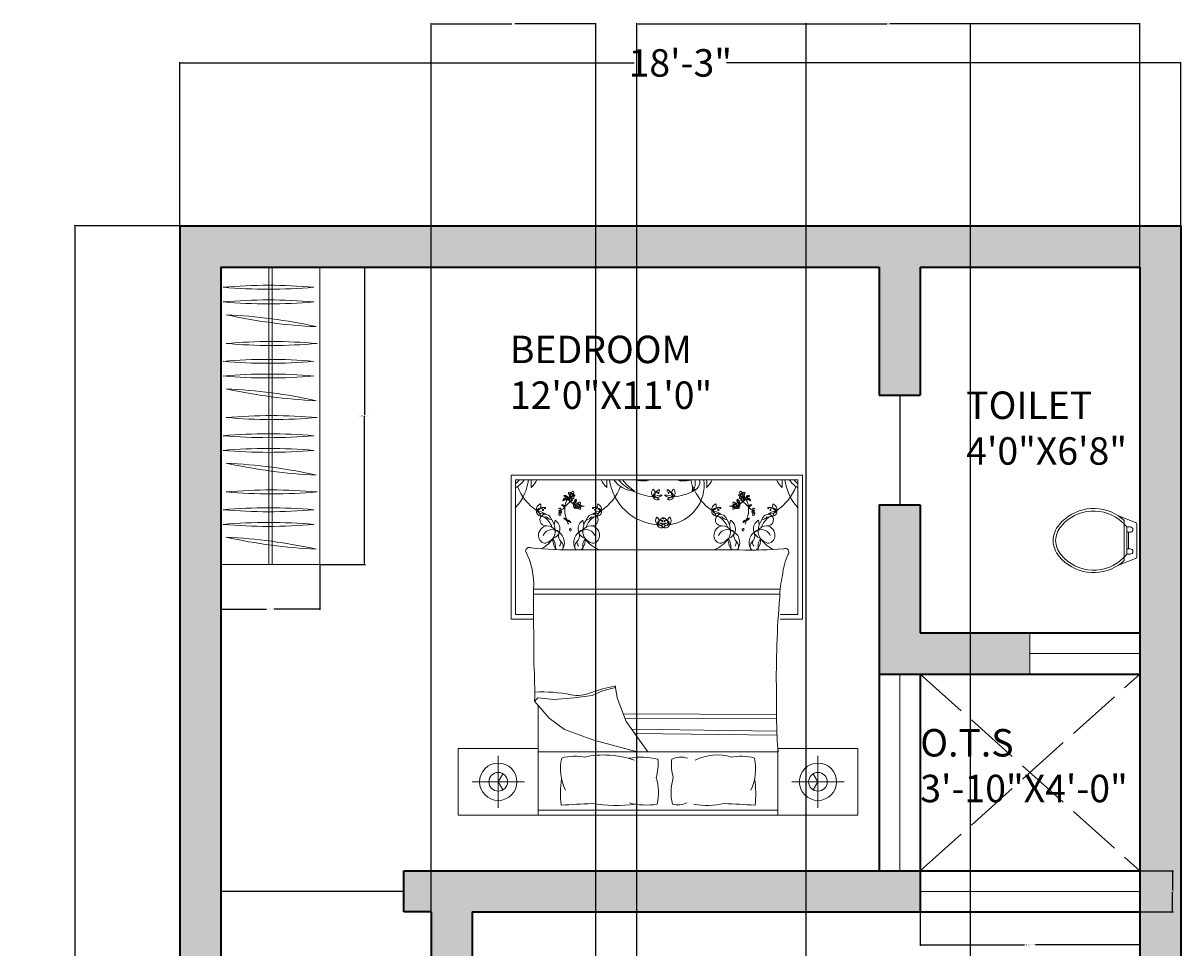
# Model space of a CAD drawing. Units: inches. Extents: x -16 to 587, y -783 to 64.
# Tile 12 of 14: x -16 to 237, y -138 to 64. Entities that reach past the tile are written whole.
import ezdxf

# ---------------------------------------------------------------- set-up
doc = ezdxf.new("R2010")
doc.units = ezdxf.units.IN
doc.header["$MEASUREMENT"] = 0
doc.linetypes.add('ACAD_ISO02W100', pattern=[15, 12, -3])
for name, color, linetype, lineweight in [('A-ANNO-DIMS', 2, 'Continuous', 18), ('A-AREA-IDEN', 7, 'Continuous', 18), ('A-DOOR', 3, 'Continuous', 25), ('A-FLOR-FIXT', 9, 'Continuous', 18), ('A-FLOR-OPEN', 8, 'ACAD_ISO02W100', 13), ('A-FURN', 8, 'Continuous', 18), ('A-GLAZ', 4, 'Continuous', 18), ('A-WALL', 7, 'Continuous', 35), ('A-WALL-PATT', 23, 'Continuous', 13)]:
    doc.layers.add(name, color=color, linetype=linetype, lineweight=lineweight)
doc.styles.get("Standard").update_dxf_attribs({"font": 'arial.ttf'})
doc.dimstyles.get("Standard").update_dxf_attribs({"dimtxt": 0.18, "dimasz": 0.18, "dimexe": 0.18, "dimexo": 0.0625, "dimgap": 0.09, "dimtad": 0, "dimtih": 1, "dimtoh": 1, "dimdec": 0, "dimzin": 0, "dimdsep": 46, "dimlunit": 3, "dimtxsty": 'Standard', "dimcen": 0.09, "dimadec": 0, "dimazin": 0, "dimtfac": 1, "dimtdec": 0, "dimtofl": 0, "dimtmove": 0, "dimatfit": 3, "dimfxl": 1, "dimtolj": 1, "dimtzin": 0, "dimarcsym": 0})

# ---------------------------------------------------------------- blocks, each defined once
blk = doc.blocks.new('*D5')
at = {"layer": 'A-ANNO-DIMS', "color": 0, "lineweight": -2, "transparency": 16777216}
for p, q in [((18.08, 19.51), (18.08, 55.27)), ((18.26, 55.09), (117.47, 55.09)), ((236.9, 55.09), (137.7, 55.09)), ((237.08, 19.51), (237.08, 55.27))]:
    blk.add_line(p, q, dxfattribs=at)
at = {"layer": 'A-ANNO-DIMS', "color": 0, "transparency": 16777216}
for points in [[(18.26, 55.12), (18.26, 55.06), (18.08, 55.09)], [(236.9, 55.12), (236.9, 55.06), (237.08, 55.09)]]:
    blk.add_solid(points, dxfattribs=at)
at = {"layer": 'Defpoints', "color": 0, "transparency": 16777216}
for p in [(237.08, 55.09), (18.08, 19.45), (237.08, 19.45)]:
    blk.add_point(p, dxfattribs=at)
at = {"layer": 'A-ANNO-DIMS', "color": 0, "transparency": 16777216, "insert": (127.58, 55.09), "char_height": 6, "attachment_point": 5}
blk.add_mtext('\\A1;18\'-3"', dxfattribs=at)
blk = doc.blocks.new('*D6')
at = {"layer": 'A-ANNO-DIMS', "color": 0, "lineweight": -2, "transparency": 16777216}
for p, q in [((18.02, 19.45), (-5.05, 19.45)), ((-4.87, 19.27), (-4.87, -355.9)), ((-4.87, -737.37), (-4.87, -362.21)), ((18.02, -737.55), (-5.05, -737.55))]:
    blk.add_line(p, q, dxfattribs=at)
at = {"layer": 'A-ANNO-DIMS', "color": 0, "transparency": 16777216}
for points in [[(-4.9, 19.27), (-4.84, 19.27), (-4.87, 19.45)], [(-4.9, -737.37), (-4.84, -737.37), (-4.87, -737.55)]]:
    blk.add_solid(points, dxfattribs=at)
at = {"layer": 'Defpoints', "color": 0, "transparency": 16777216}
for p in [(18.08, 19.45), (-4.87, -737.55), (18.08, -737.55)]:
    blk.add_point(p, dxfattribs=at)
at = {"layer": 'A-ANNO-DIMS', "color": 0, "transparency": 16777216, "insert": (-4.87, -359.05), "char_height": 6, "attachment_point": 5}
blk.add_mtext('\\A1;63\'-1"', dxfattribs=at)
blk = doc.blocks.new('BED-DOUBLE-LARGE')
for p, q in [((11.54, 74.35), (11.54, 42.86)), ((75.28, 74.35), (11.54, 74.35)), ((75.28, 42.86), (75.28, 74.35)), ((12.55, 73.34), (74.26, 73.34)), ((12.55, 43.87), (12.55, 73.34)), ((74.26, 73.34), (74.26, 43.87)), ((21.17, 64.47), (20.98, 63.49)), ((27.28, 64.47), (27.47, 63.49)), ((59.54, 64.47), (59.35, 63.49)), ((65.65, 64.47), (65.84, 63.49)), ((61.46, 57.99), (25.97, 57.99)), ((70.42, 49.4), (16.48, 49.4)), ((70.34, 48.31), (16.48, 48.31)), ((16.48, 43.87), (12.55, 43.87)), ((74.26, 43.87), (70.41, 43.87)), ((11.54, 42.86), (16.49, 42.86)), ((70.43, 42.86), (75.28, 42.86)), ((34.41, 27.92), (31.58, 27.21)), ((34.77, 25.62), (34.41, 27.92)), ((17.41, 25.62), (16.7, 24.91)), ((20.95, 25.26), (17.41, 25.62)), ((25.38, 25.62), (20.95, 25.26)), ((29.28, 26.15), (25.38, 25.62)), ((31.58, 27.21), (29.28, 26.15)), ((36.71, 20.49), (34.77, 25.62)), ((16.7, 24.91), (19.89, 21.19)), ((17.49, 0), (17.49, 24)), ((19.89, 21.19), (23.25, 18.72)), ((69.63, 22), (36.09, 22.13)), ((69.63, 21.1), (36.43, 21.23)), ((41.5, 13.82), (36.71, 20.49)), ((23.25, 18.72), (29.63, 16.41)), ((69.67, 18.35), (37.93, 18.79)), ((69.71, 17.45), (38.58, 17.88)), ((29.63, 16.41), (39.16, 13.82)), ((8.74, 13), (8.74, 1.57)), ((17.49, 13.82), (69.94, 13.82)), ((78.68, 13), (78.68, 1.57)), ((14.46, 7.29), (3.03, 7.29)), ((72.97, 7.29), (84.4, 7.29)), ((0, 0), (87.43, 0)), ((69.94, 1.12), (17.49, 1.12))]:
    blk.add_line(p, q)
for points in [[(16.52, 32.91, -0.001242), (16.48, 49.5, 0.127202), (14.73, 57.77)], [(70.32, 47.62, -0.056112), (70.95, 52.43, -0.095341), (72.18, 57.07)], [(22.51, 2.18, -0.074897), (22.61, 7.89, 0.472817)], [(43.3, 8.21, -0.14099), (43.48, 2.38, -0.235245)], [(47.04, 8.21, 0.14099), (46.86, 2.38, 0.235245)], [(64.92, 2.18, 0.074897), (64.81, 7.89, -0.472817)]]:
    blk.add_lwpolyline(points, format="xyb")
for points in [[(17.49, 14.57), (0, 14.57), (0, 0)], [(69.94, 0), (69.94, 14.57), (87.43, 14.57), (87.43, 0)], [(8.74, 7.29), (9.76, 9.05)], [(78.68, 7.29), (77.66, 9.05)], [(8.74, 7.29), (9.76, 5.52)], [(78.68, 7.29), (77.66, 5.52)]]:
    blk.add_lwpolyline(points)
for centre, radius in [((24.76, 69.99), 0.223), ((62.05, 69.99), 0.223), ((26.22, 67.64), 0.223), ((60.6, 67.64), 0.223), ((8.74, 7.29), 4.08), ((78.68, 7.29), 4.08), ((8.74, 7.29), 2.04), ((78.68, 7.29), 2.04)]:
    blk.add_circle(centre, radius)
for centre, radius, start, end in [((7.78, 77.44), 6.93, 313.5186, 323.6964), ((9.78, 76.41), 5.56, 299.8884, 326.5383), ((4.05, 74.88), 11.42, 318.1144, 352.255), ((23.59, 76.01), 11.42, 201.4092, 235.6135), ((12.9, 75.12), 4.64, 311.0454, 337.4453), ((0.18, 72.62), 15.8, 356.3481, 2.5919), ((35.55, 75.12), 4.64, 202.5547, 228.9546), ((24.86, 76.01), 11.42, 304.3865, 338.5908), ((48.27, 72.62), 15.8, 177.4081, 183.6519), ((44.39, 74.88), 11.42, 187.745, 265.5377), ((38.67, 76.41), 5.56, 213.4617, 268.728), ((40.67, 77.44), 6.93, 216.3036, 252.1496), ((44.31, 79.39), 10.31, 215.947, 235.9877), ((40.33, 79.34), 6.28, 252.9798, 286.4569), ((42.81, 82.58), 9.28, 264.3643, 265.6213), ((47.7, 88.94), 16.59, 250.0972, 250.2783), ((43.57, 70.46), 1.27, 140.8855, 222.2127), ((42.13, 70.42), 0.953, 301.6373, 61.4609), ((45.36, 68.67), 2.89, 121.989, 161.0841), ((43.91, 71), 0.142, 288.4408, 121.989), ((43.93, 70.93), 0.0689, 171.9833, 288.4408), ((45.82, 71), 0.142, 58.011, 251.5592), ((45.8, 70.93), 0.0689, 251.5592, 8.0167), ((44.37, 68.67), 2.89, 18.9159, 58.011), ((44.97, 72.24), 8.84, 278.1803, 7.1364), ((47.6, 70.42), 0.953, 118.5391, 238.3627), ((46.16, 70.46), 1.27, 317.7873, 39.1145), ((49.41, 79.34), 6.28, 253.5431, 287.0202), ((46.92, 82.58), 9.28, 274.3787, 275.6357), ((42.03, 88.94), 16.59, 289.7217, 289.9028), ((46.11, 71.43), 5.11, 353.3805, 21.883), ((50.8, 72.86), 2.05, 280.9261, 13.6102), ((49.26, 72.57), 2.59, 318.0951, 17.1391), ((61.96, 76.01), 11.42, 201.4092, 235.6135), ((38.55, 72.62), 15.8, 356.3481, 2.5919), ((51.27, 75.12), 4.64, 311.0454, 337.4453), ((73.92, 75.12), 4.64, 202.5547, 228.9546), ((63.23, 76.01), 11.42, 304.3865, 338.5908), ((86.64, 72.62), 15.8, 177.4081, 183.6519), ((82.76, 74.88), 11.42, 187.745, 221.8856), ((77.04, 76.41), 5.56, 213.4617, 240.1116), ((79.04, 77.44), 6.93, 216.3036, 226.4814), ((23.14, 68.85), 0.249, 123.0979, 213.1364), ((23.57, 68.49), 0.673, 92.3172, 160.5201), ((26.65, 63.38), 6.5, 121.1156, 124.8118), ((23.49, 68.75), 0.58, 82.6008, 147.1845), ((23.33, 69.66), 0.249, 55.6077, 145.6462), ((23.16, 69.13), 0.673, 21.7087, 93.0299), ((19.61, 64.33), 6.5, 53.6254, 57.3216), ((23.42, 68.72), 0.257, 45.7354, 121.1156), ((26.93, 67.08), 3.63, 150.7959, 175.244), ((32.15, 59.35), 11.95, 127.8256, 137.7588), ((23.36, 69.3), 0.58, 342.8042, 79.6943), ((23.31, 69.36), 0.257, 338.2452, 53.6254), ((23.73, 69.19), 0.194, 158.2452, 340.6395), ((23.74, 69.05), 0.194, 225.7354, 48.1297), ((27.39, 70.82), 3.88, 201.7087, 206.2181), ((24.3, 68.17), 1.01, 40.9365, 112.7695), ((23.96, 68.51), 0.597, 49.3812, 95.5456), ((26.93, 67.08), 3.63, 137.5083, 145.9967), ((24.4, 68.75), 0.617, 61.1838, 141.6792), ((27.3, 71.9), 4.35, 220.182, 239.456), ((24.3, 70.41), 0.221, 134.3732, 211.9501), ((24.7, 70.66), 0.702, 211.9501, 255.2442), ((24.31, 70.16), 0.439, 8.5614, 112.5914), ((24.52, 69.68), 0.304, 88.5719, 233.8954), ((24.48, 69.6), 0.218, 228.2946, 6.2474), ((24.82, 69.51), 0.718, 229.3812, 289.9959), ((24.43, 70.18), 0.147, 352.868, 97.094), ((24.28, 69.86), 0.306, 298.8493, 359.9355), ((24.35, 69.6), 0.35, 4.2123, 48.1587), ((25.07, 70.4), 0.368, 100.9597, 208.7804), ((25.07, 69.64), 0.371, 183.635, 258.4363), ((24.36, 68.63), 0.737, 15.6484, 62.2957), ((25.02, 69.78), 0.213, 178.1325, 268.8919), ((25.46, 69.91), 0.676, 132.3896, 156.5724), ((25.17, 69.83), 0.364, 42.3208, 130.2111), ((25.25, 70.21), 0.46, 226.3462, 279.6513), ((24.77, 69.35), 0.535, 7.4968, 71.2737), ((24.76, 70.6), 0.517, 291.6382, 4.947), ((25.16, 70.68), 0.729, 254.2829, 276.9148), ((25.1, 70.63), 0.171, 4.947, 127.5263), ((25.14, 69.38), 0.172, 215.0752, 14.7644), ((24.78, 69.11), 1.01, 287.889, 359.722), ((24.75, 68.64), 0.597, 305.1128, 351.2773), ((25.23, 68.74), 0.617, 271.4625, 339.4747), ((25.29, 69.94), 0.192, 279.6513, 42.3208), ((26.05, 68.44), 0.718, 110.6625, 171.2773), ((25.13, 68.8), 0.737, 338.3627, 25.0101), ((26.52, 68.05), 0.368, 100.9597, 208.7804), ((26.56, 68.28), 0.171, 4.947, 127.5263), ((43.52, 80.99), 11.42, 242.5854, 265.5377), ((43.56, 69.65), 0.934, 76.148, 182.2415), ((45.02, 61.99), 7.99, 92.7418, 107.407), ((43.37, 71.25), 1.8, 245.6899, 314.4589), ((42.58, 67.66), 1.95, 44.6273, 88.5415), ((43.54, 69.87), 0.946, 196.1963, 296.9726), ((43.76, 70.43), 0.123, 140.0755, 76.148), ((44.71, 61.99), 7.99, 72.593, 87.2582), ((46.36, 71.25), 1.8, 225.5411, 294.3101), ((47.15, 67.66), 1.95, 91.4585, 135.3727), ((46.19, 69.87), 0.946, 243.0274, 343.8037), ((45.96, 70.39), 0.0744, 103.9791, 39.8091), ((46.17, 69.65), 0.934, 357.7585, 103.852), ((46.21, 80.99), 11.42, 274.4623, 297.4146), ((60.26, 68.28), 0.171, 52.4737, 175.053), ((60.3, 68.05), 0.368, 331.2196, 79.0403), ((61.69, 68.8), 0.737, 154.9899, 201.6373), ((61.58, 68.74), 0.617, 200.5253, 268.5375), ((62.04, 69.11), 1.01, 180.278, 252.111), ((60.77, 68.44), 0.718, 8.7227, 69.3375), ((61.52, 69.94), 0.192, 137.6792, 260.3487), ((61.65, 69.83), 0.364, 49.7889, 137.6792), ((62.07, 68.64), 0.597, 188.7227, 234.8872), ((61.57, 70.21), 0.46, 260.3487, 313.6538), ((62.05, 69.35), 0.535, 108.7263, 172.5032), ((61.68, 69.38), 0.172, 165.2356, 324.9248), ((61.72, 70.63), 0.171, 52.4737, 175.053), ((62.06, 70.6), 0.517, 175.053, 248.3618), ((61.66, 70.68), 0.729, 263.0852, 285.7171), ((59.52, 71.9), 4.35, 300.544, 319.818), ((62.46, 68.63), 0.737, 117.7043, 164.3516), ((62.52, 68.17), 1.01, 67.2305, 139.0635), ((62, 69.51), 0.718, 250.0041, 310.6188), ((61.8, 69.78), 0.213, 271.1081, 1.8675), ((61.35, 69.91), 0.676, 23.4276, 47.6104), ((61.75, 70.4), 0.368, 331.2196, 79.0403), ((61.75, 69.64), 0.371, 281.5637, 356.365), ((54.66, 59.35), 11.95, 42.2412, 52.1744), ((62.51, 70.16), 0.439, 67.4086, 171.4386), ((62.47, 69.6), 0.35, 131.8413, 175.7877), ((62.33, 69.6), 0.218, 173.7526, 311.7054), ((62.42, 68.75), 0.617, 38.3208, 118.8162), ((62.54, 69.86), 0.306, 180.0645, 241.1507), ((62.38, 70.18), 0.147, 82.906, 187.132), ((62.11, 70.66), 0.702, 284.7558, 328.0499), ((62.3, 69.68), 0.304, 306.1046, 91.4281), ((62.85, 68.51), 0.597, 84.4544, 130.6188), ((59.89, 67.08), 3.63, 34.0033, 42.4917), ((62.52, 70.41), 0.221, 328.0499, 45.6268), ((63.45, 69.3), 0.58, 100.3057, 197.1958), ((63.08, 69.05), 0.194, 131.8703, 314.2646), ((63.08, 69.19), 0.194, 199.3605, 21.7548), ((59.43, 70.82), 3.88, 333.7819, 338.2913), ((63.66, 69.13), 0.673, 86.9701, 158.2913), ((59.89, 67.08), 3.63, 4.756, 29.2041), ((63.4, 68.72), 0.257, 58.8844, 134.2646), ((63.5, 69.36), 0.257, 126.3746, 201.7548), ((63.32, 68.75), 0.58, 32.8155, 97.3992), ((63.25, 68.49), 0.673, 19.4799, 87.6828), ((63.49, 69.66), 0.249, 34.3538, 124.3923), ((67.21, 64.33), 6.5, 122.6784, 126.3746), ((60.17, 63.38), 6.5, 55.1882, 58.8844), ((63.67, 68.85), 0.249, 326.8636, 56.9021), ((18.37, 66.85), 1.27, 110.9613, 192.2885), ((18.06, 66.36), 0.946, 166.272, 267.0484), ((17.11, 67.54), 0.953, 271.7131, 31.5367), ((19.04, 64.41), 2.89, 92.0648, 131.1598), ((17.96, 66.15), 0.934, 46.2238, 152.3173), ((15.41, 58.79), 7.99, 62.8176, 77.4827), ((18.6, 67.64), 1.8, 215.7657, 284.5347), ((16.12, 64.92), 1.95, 14.7031, 58.6173), ((18.53, 66.74), 0.123, 110.2817, 46.2238), ((18.92, 67.08), 0.0689, 142.0591, 258.5166), ((18.94, 67.15), 0.142, 258.5166, 92.0648), ((22.21, 66.73), 0.368, 100.9597, 142.2379), ((21.9, 66.32), 0.223, 273.2768, 86.7232), ((22.16, 66.11), 0.213, 178.1325, 268.8919), ((22.6, 66.24), 0.676, 132.3896, 156.5724), ((22.31, 66.16), 0.364, 42.3208, 130.2111), ((22.39, 66.54), 0.46, 226.3462, 279.6513), ((21.91, 65.68), 0.535, 7.4968, 71.2737), ((21.9, 66.93), 0.517, 291.6382, 4.947), ((22.3, 67.01), 0.729, 254.2829, 276.9148), ((22.24, 66.96), 0.171, 4.947, 127.5263), ((17.25, 73.06), 8.3, 307.9541, 316.8459), ((22.43, 66.27), 0.192, 279.6513, 42.3208), ((22.65, 65.38), 2.47, 82.8698, 91.6736), ((22.99, 68.05), 0.459, 205.5379, 258.6744), ((22.33, 66.49), 1.38, 59.344, 79.7412), ((22.03, 66.49), 1.4, 43.6929, 51.7899), ((22.89, 67.42), 0.42, 355.7131, 81.6568), ((22.66, 67.05), 0.733, 27.3659, 59.344), ((23.21, 67.53), 0.178, 202.5583, 304.2343), ((30.53, 66.9), 7.24, 176.1723, 196.4158), ((25.06, 67.54), 0.617, 3.8774, 87.1501), ((24.62, 67.78), 0.597, 352.0748, 38.2393), ((24.52, 67.31), 1.01, 343.6301, 55.4631), ((25.92, 67.6), 0.718, 172.0748, 232.6895), ((24.94, 67.52), 0.737, 318.342, 4.9894), ((25.75, 68.06), 0.221, 134.3732, 211.9501), ((27.3, 71.9), 4.35, 246.1523, 246.9499), ((26.16, 68.32), 0.702, 211.9501, 255.2442), ((25.77, 67.81), 0.439, 8.5614, 112.5914), ((25.97, 67.33), 0.304, 88.5719, 233.8954), ((25.94, 67.25), 0.218, 228.2946, 6.2474), ((25.89, 67.83), 0.147, 352.868, 97.094), ((25.73, 67.51), 0.306, 298.8493, 359.9355), ((25.81, 67.25), 0.35, 4.2123, 48.1587), ((26.53, 67.3), 0.371, 183.635, 258.4363), ((26.48, 67.43), 0.213, 178.1325, 268.8919), ((26.92, 67.57), 0.676, 132.3896, 156.5724), ((26.62, 67.48), 0.364, 42.3208, 130.2111), ((26.7, 67.86), 0.46, 226.3462, 279.6513), ((26.21, 68.25), 0.517, 291.6382, 4.947), ((26.23, 67.01), 0.535, 7.4968, 71.2737), ((26.62, 68.34), 0.729, 254.2829, 276.9148), ((26.59, 67.03), 0.172, 215.0752, 14.7644), ((26.75, 67.59), 0.192, 279.6513, 42.3208), ((27.3, 71.9), 4.35, 265.2415, 272.8929), ((29.51, 67.15), 0.142, 87.9352, 281.4834), ((29.84, 67.64), 1.8, 255.4653, 324.2343), ((33.04, 58.79), 7.99, 102.5173, 117.1824), ((29.41, 64.41), 2.89, 48.8402, 87.9352), ((29.52, 67.08), 0.0689, 281.4834, 37.9409), ((30.48, 66.15), 0.934, 27.6827, 133.7762), ((29.94, 66.69), 0.0744, 133.7729, 69.7333), ((31.34, 67.54), 0.953, 148.4633, 268.2869), ((30.39, 66.36), 0.946, 272.9516, 13.728), ((32.32, 64.92), 1.95, 121.3827, 165.2969), ((30.07, 66.85), 1.27, 347.7115, 69.0387), ((56.75, 66.85), 1.27, 110.9613, 192.2885), ((56.43, 66.36), 0.946, 166.272, 267.0484), ((55.48, 67.54), 0.953, 271.7131, 31.5367), ((57.41, 64.41), 2.89, 92.0648, 131.1598), ((56.34, 66.15), 0.934, 46.2238, 152.3173), ((54.49, 64.92), 1.95, 14.7031, 58.6173), ((56.97, 67.64), 1.8, 215.7657, 284.5347), ((53.78, 58.79), 7.99, 62.8176, 77.4827), ((56.9, 66.74), 0.123, 110.2817, 46.2238), ((57.3, 67.08), 0.0689, 142.0591, 258.5166), ((57.31, 67.15), 0.142, 258.5166, 92.0648), ((59.52, 71.9), 4.35, 267.1071, 274.7585), ((60.07, 67.59), 0.192, 137.6792, 260.3487), ((60.2, 67.48), 0.364, 49.7889, 137.6792), ((60.11, 67.86), 0.46, 260.3487, 313.6538), ((60.22, 67.03), 0.172, 165.2356, 324.9248), ((60.59, 67.01), 0.535, 108.7263, 172.5032), ((60.61, 68.25), 0.517, 175.053, 248.3618), ((60.2, 68.34), 0.729, 263.0852, 285.7171), ((60.34, 67.43), 0.213, 271.1081, 1.8675), ((59.9, 67.57), 0.676, 23.4276, 47.6104), ((60.29, 67.3), 0.371, 281.5637, 356.365), ((61.05, 67.81), 0.439, 67.4086, 171.4386), ((61.01, 67.25), 0.35, 131.8413, 175.7877), ((60.88, 67.25), 0.218, 173.7526, 311.7054), ((60.93, 67.83), 0.147, 82.906, 187.132), ((61.08, 67.51), 0.306, 180.0645, 241.1507), ((60.66, 68.32), 0.702, 284.7558, 328.0499), ((60.84, 67.33), 0.304, 306.1046, 91.4281), ((61.88, 67.52), 0.737, 175.0106, 221.658), ((61.76, 67.54), 0.617, 92.8499, 176.1226), ((61.07, 68.06), 0.221, 328.0499, 45.6268), ((59.52, 71.9), 4.35, 293.0501, 293.8477), ((62.3, 67.31), 1.01, 124.5369, 196.3699), ((60.89, 67.6), 0.718, 307.3105, 7.9252), ((62.2, 67.78), 0.597, 141.7607, 187.9252), ((56.28, 66.9), 7.24, 343.5842, 3.8277), ((63.93, 67.42), 0.42, 98.3432, 184.2869), ((64.16, 67.05), 0.733, 120.656, 152.6341), ((63.61, 67.53), 0.178, 235.7657, 337.4417), ((69.56, 73.06), 8.3, 223.1541, 232.0459), ((64.79, 66.49), 1.4, 128.2101, 136.3071), ((64.49, 66.49), 1.38, 100.2588, 120.656), ((64.17, 65.38), 2.47, 88.3264, 97.1302), ((63.83, 68.05), 0.459, 281.3256, 334.4621), ((64.38, 66.27), 0.192, 137.6792, 260.3487), ((64.51, 66.16), 0.364, 49.7889, 137.6792), ((64.43, 66.54), 0.46, 260.3487, 313.6538), ((64.9, 65.68), 0.535, 108.7263, 172.5032), ((64.58, 66.96), 0.171, 52.4737, 175.053), ((64.92, 66.93), 0.517, 175.053, 248.3618), ((64.52, 67.01), 0.729, 263.0852, 285.7171), ((64.66, 66.11), 0.213, 271.1081, 1.8675), ((64.21, 66.24), 0.676, 23.4276, 47.6104), ((64.61, 66.73), 0.368, 37.7621, 79.0403), ((64.91, 66.32), 0.223, 93.2768, 266.7232), ((67.88, 67.15), 0.142, 87.9352, 281.4834), ((71.41, 58.79), 7.99, 102.5173, 117.1824), ((68.22, 67.64), 1.8, 255.4653, 324.2343), ((67.78, 64.41), 2.89, 48.8402, 87.9352), ((67.89, 67.08), 0.0689, 281.4834, 37.9409), ((68.85, 66.15), 0.934, 27.6827, 133.7762), ((68.31, 66.69), 0.0744, 133.7729, 69.7333), ((69.71, 67.54), 0.953, 148.4633, 268.2869), ((70.7, 64.92), 1.95, 121.3827, 165.2969), ((68.76, 66.36), 0.946, 272.9516, 13.728), ((68.44, 66.85), 1.27, 347.7115, 69.0387), ((19.17, 64.55), 1.31, 109.1312, 279.736), ((18.9, 65.97), 0.804, 216.7319, 296.0245), ((16.57, 61.66), 4.13, 18.2955, 58.7386), ((18.85, 64.15), 1.64, 15.6955, 94.031), ((20.62, 66.33), 1.75, 218.4175, 263.8338), ((16.53, 61.99), 4.69, 3.4924, 33.7117), ((20.08, 62.59), 2.17, 286.8663, 60.0915), ((22.21, 65.97), 0.371, 217.3642, 258.4363), ((22.28, 65.71), 0.172, 215.0752, 14.7644), ((23.17, 62.44), 2.47, 82.8698, 91.6736), ((23.51, 65.1), 0.459, 205.5379, 258.6744), ((22.85, 63.55), 1.38, 59.344, 79.7412), ((22.55, 63.55), 1.4, 43.6929, 51.7899), ((23.41, 64.47), 0.42, 355.7131, 81.6568), ((23.18, 64.11), 0.733, 27.3659, 59.344), ((23.73, 64.59), 0.178, 202.5583, 304.2343), ((30.53, 66.9), 7.24, 200.1059, 206.9968), ((24.06, 64.09), 0.42, 36.5232, 122.4668), ((23.84, 63.71), 0.733, 58.836, 90.8141), ((24.01, 64.42), 0.178, 173.9457, 275.6216), ((23.65, 62.89), 1.4, 66.3901, 74.4871), ((24.57, 64.47), 0.459, 219.5056, 272.6421), ((23.5, 63.15), 1.38, 38.4388, 58.836), ((22.38, 62.91), 2.47, 26.5064, 35.3102), ((28.36, 62.59), 2.17, 119.9085, 253.1337), ((31.92, 61.99), 4.69, 146.2883, 176.5076), ((31.88, 61.66), 4.13, 121.2614, 161.7045), ((29.59, 64.15), 1.64, 85.969, 164.3045), ((27.83, 66.33), 1.75, 276.1662, 321.5825), ((29.28, 64.55), 1.31, 260.264, 70.8688), ((29.55, 65.97), 0.804, 243.9755, 323.2681), ((44.44, 64.35), 1.27, 140.8855, 222.2127), ((43.01, 64.31), 0.953, 301.6373, 61.4609), ((44.44, 63.53), 0.934, 76.148, 182.2415), ((46.24, 62.56), 2.89, 121.989, 161.0841), ((44.25, 65.14), 1.8, 245.6899, 314.4589), ((45.89, 55.87), 7.99, 92.7418, 107.407), ((44.41, 63.76), 0.946, 196.1963, 296.9726), ((43.46, 61.55), 1.95, 44.6273, 88.5415), ((45.48, 65.14), 1.8, 225.5411, 294.3101), ((43.84, 55.87), 7.99, 72.593, 87.2582), ((44.63, 64.32), 0.123, 140.0755, 76.148), ((44.78, 64.89), 0.142, 288.4408, 121.989), ((44.81, 64.82), 0.0689, 171.9833, 288.4408), ((44.95, 64.89), 0.142, 58.011, 251.5592), ((45.32, 63.76), 0.946, 243.0274, 343.8037), ((46.28, 61.55), 1.95, 91.4585, 135.3727), ((44.93, 64.82), 0.0689, 251.5592, 8.0167), ((45.09, 64.27), 0.0744, 103.9791, 39.8091), ((43.5, 62.56), 2.89, 18.9159, 58.011), ((45.29, 63.53), 0.934, 357.7585, 103.852), ((46.73, 64.31), 0.953, 118.5391, 238.3627), ((45.29, 64.35), 1.27, 317.7873, 39.1145), ((57.54, 64.55), 1.31, 109.1312, 279.736), ((57.27, 65.97), 0.804, 216.7319, 296.0245), ((54.94, 61.66), 4.13, 18.2955, 58.7386), ((57.22, 64.15), 1.64, 15.6955, 94.031), ((58.99, 66.33), 1.75, 218.4175, 263.8338), ((54.9, 61.99), 4.69, 3.4924, 33.7117), ((58.46, 62.59), 2.17, 286.8663, 60.0915), ((63.31, 63.15), 1.38, 121.164, 141.5612), ((64.44, 62.91), 2.47, 144.6898, 153.4936), ((62.25, 64.47), 0.459, 267.3579, 320.4944), ((62.76, 64.09), 0.42, 57.5332, 143.4768), ((62.98, 63.71), 0.733, 89.1859, 121.164), ((63.17, 62.89), 1.4, 105.5129, 113.6099), ((56.28, 66.9), 7.24, 333.0032, 339.8941), ((62.81, 64.42), 0.178, 264.3784, 6.0543), ((63.41, 64.47), 0.42, 98.3432, 184.2869), ((63.64, 64.11), 0.733, 120.656, 152.6341), ((63.09, 64.59), 0.178, 235.7657, 337.4417), ((64.27, 63.55), 1.4, 128.2101, 136.3071), ((63.97, 63.55), 1.38, 100.2588, 120.656), ((63.65, 62.44), 2.47, 88.3264, 97.1302), ((63.31, 65.1), 0.459, 281.3256, 334.4621), ((64.54, 65.71), 0.172, 165.2356, 324.9248), ((66.73, 62.59), 2.17, 119.9085, 253.1337), ((64.61, 65.97), 0.371, 281.5637, 322.6358), ((70.29, 61.99), 4.69, 146.2883, 176.5076), ((70.25, 61.66), 4.13, 121.2614, 161.7045), ((67.96, 64.15), 1.64, 85.969, 164.3045), ((66.2, 66.33), 1.75, 276.1662, 321.5825), ((67.65, 64.55), 1.31, 260.264, 70.8688), ((67.92, 65.97), 0.804, 243.9755, 323.2681), ((19.65, 61.18), 2.09, 97.1143, 185.0551), ((19.04, 60.97), 1.48, 178.9462, 275.5144), ((20.47, 60.39), 2.03, 68.5779, 158.4181), ((18.59, 62.06), 2.63, 283.079, 4.7067), ((19.29, 60.71), 2.54, 35.9599, 87.6409), ((24.06, 60.21), 3.37, 143.6555, 147.2989), ((21.46, 61.68), 0.543, 344.8529, 102.6959), ((20.42, 59.58), 2.79, 330.8249, 70.7178), ((23.71, 61.07), 1.79, 164.8529, 228.4347), ((24.47, 62.5), 0.169, 79.5616, 257.2949), ((24.46, 62.4), 0.274, 259.5864, 79.5616), ((28.03, 59.58), 2.79, 109.2822, 209.1751), ((24.73, 61.07), 1.79, 311.5653, 15.1471), ((26.99, 61.68), 0.543, 77.3041, 195.1471), ((29.16, 60.71), 2.54, 92.3591, 144.0401), ((24.39, 60.21), 3.37, 32.7011, 36.3445), ((29.86, 62.06), 2.63, 175.2933, 256.921), ((27.98, 60.39), 2.03, 21.5819, 111.4221), ((28.8, 61.18), 2.09, 354.9449, 82.8857), ((29.4, 60.97), 1.48, 264.4856, 1.0538), ((58.02, 61.18), 2.09, 97.1143, 185.0551), ((57.41, 60.97), 1.48, 178.9462, 275.5144), ((58.84, 60.39), 2.03, 68.5779, 158.4181), ((56.96, 62.06), 2.63, 283.079, 4.7067), ((57.66, 60.71), 2.54, 35.9599, 87.6409), ((62.43, 60.21), 3.37, 143.6555, 147.2989), ((59.83, 61.68), 0.543, 344.8529, 102.6959), ((58.79, 59.58), 2.79, 330.8249, 70.7178), ((62.09, 61.07), 1.79, 164.8529, 228.4347), ((62.36, 62.4), 0.274, 100.4384, 280.4136), ((62.34, 62.5), 0.169, 282.7051, 100.4384), ((66.4, 59.58), 2.79, 109.2822, 209.1751), ((63.1, 61.07), 1.79, 311.5653, 15.1471), ((65.36, 61.68), 0.543, 77.3041, 195.1471), ((67.53, 60.71), 2.54, 92.3591, 144.0401), ((62.76, 60.21), 3.37, 32.7011, 36.3445), ((68.23, 62.06), 2.63, 175.2933, 256.921), ((66.35, 60.39), 2.03, 21.5819, 111.4221), ((67.17, 61.18), 2.09, 354.9449, 82.8857), ((67.77, 60.97), 1.48, 264.4856, 1.0538), ((15.53, 57.71), 0.807, 62.6588, 176.02), ((24.92, 148.99), 91.01, 264.3113, 270.6567), ((15.19, 64.15), 6.62, 296.7003, 326.3329), ((24.06, 60.21), 3.37, 175.2696, 214.215), ((17.62, 58.64), 3.62, 350.8446, 31.1782), ((22.1, 58.96), 1.05, 217.675, 239.9707), ((20, 60.08), 2.51, 330.0851, 352.564), ((21.66, 58.75), 1.31, 336.1646, 48.4347), ((26.79, 58.75), 1.31, 131.5653, 203.8354), ((28.45, 60.08), 2.51, 187.436, 209.9149), ((26.34, 58.96), 1.05, 293.2856, 322.325), ((24.39, 60.21), 3.37, 325.785, 4.7304), ((30.83, 58.64), 3.62, 148.8218, 190.2867), ((33.26, 64.15), 6.62, 213.6671, 248.5059), ((53.56, 64.15), 6.62, 291.4941, 326.3329), ((62.43, 60.21), 3.37, 175.2696, 214.215), ((55.99, 58.64), 3.62, 349.7133, 31.1782), ((60.47, 58.96), 1.05, 217.675, 246.7144), ((58.37, 60.08), 2.51, 330.0851, 352.564), ((60.03, 58.75), 1.31, 336.1646, 48.4347), ((65.16, 58.75), 1.31, 131.5653, 203.8354), ((66.82, 60.08), 2.51, 187.436, 209.9149), ((64.72, 58.96), 1.05, 287.4186, 322.325), ((62.76, 60.21), 3.37, 325.785, 4.7304), ((69.2, 58.64), 3.62, 148.8218, 190.751), ((71.63, 64.15), 6.62, 213.6671, 246.3547), ((71.52, 57.51), 0.797, 326.1736, 113.4781), ((22.1, 58.96), 1.05, 296.442, 315.5483), ((26.34, 58.96), 1.05, 224.4517, 246.771), ((60.47, 58.96), 1.05, 293.2856, 315.5483), ((64.14, 143.02), 85.07, 268.1965, 274.7598), ((64.72, 58.96), 1.05, 224.4517, 253.3657), ((274.49, 30.21), 204.92, 175.1265, 180.8855), ((-63.46, 27.08), 80.19, 358.447, 4.1706), ((40.48, -5.12), 33.91, 100.6617, 109.8806), ((34.21, 27.99), 0.211, 340.2464, 91.1377), ((18.2, -6.05), 33, 78.6608, 92.5481), ((26.09, 33.28), 7.12, 258.6608, 293.7384), ((226.67, 24.5), 157.09, 179.0718, 183.9), ((25.63, 1.16), 11.72, 78.9631, 104.8961), ((31.79, -7.17), 20.32, 70.7385, 101.9603), ((40.02, -2.74), 15.42, 76.3762, 100.1383), ((48.65, 8.05), 4.63, 71.4593, 114.9817), ((56.75, 2.02), 11.13, 73.8254, 116.1239), ((61.8, 1.16), 11.72, 75.1039, 101.0369), ((33.65, 10.18), 11.27, 168.2417, 204.8684), ((33, 11.13), 10.71, 344.1707, 5.9871), ((57.34, 11.13), 10.71, 174.0129, 195.8293), ((53.78, 10.18), 11.27, 335.1316, 11.7583), ((70.7, -829.84), 833.41, 92.85022, 93.31479), ((34.49, 33.82), 31.71, 260.503, 277.7804), ((41.18, 17.79), 15.58, 256.04, 278.4751), ((48.06, 6.54), 4.32, 253.8974, 296.6563), ((54.54, 17.48), 15.37, 258.8159, 283.6573), ((16.73, -829.84), 833.41, 86.68521, 87.14978)]:
    blk.add_arc(centre, radius, start, end)
blk = doc.blocks.new('WARDROBE')
for p, q in [((0, 0), (0, 65.01)), ((21.67, 65.01), (0, 65.01)), ((10.47, 0), (10.47, 65.01)), ((11.19, 0), (11.19, 65.01)), ((21.67, 0), (21.67, 65.01)), ((21.67, 0), (0, 0))]:
    blk.add_line(p, q)
for centre, start, end in [((10.4, -52.98), 85.0028, 94.9972), ((10.4, 174.18), 265.0028, 274.9972), ((10.4, -56.19), 85.0028, 94.9972), ((10.4, 170.97), 265.0028, 274.9972), ((25.83, 165.89), 257.508, 267.5023), ((-3.8, -59.33), 77.508, 87.5023), ((11.1, -65.28), 85.0028, 94.9972), ((11.1, 161.88), 265.0028, 274.9972), ((10.4, -69.18), 85.0028, 94.9972), ((10.4, 157.98), 265.0028, 274.9972), ((10.4, -72.39), 85.0028, 94.9972), ((10.4, 154.77), 265.0028, 274.9972), ((25.83, 149.7), 257.508, 267.5023), ((-3.8, -75.52), 77.508, 87.5023), ((11.1, -81.47), 85.0028, 94.9972), ((11.1, 145.69), 265.0028, 274.9972), ((10.4, -85.44), 85.0028, 94.9972), ((10.4, 141.72), 265.0028, 274.9972), ((10.4, -88.65), 85.0028, 94.9972), ((10.4, 138.51), 265.0028, 274.9972), ((-3.8, -91.78), 77.508, 87.5023), ((25.83, 133.44), 257.508, 267.5023), ((11.1, -97.73), 85.0028, 94.9972), ((11.1, 129.43), 265.0028, 274.9972), ((10.4, -101.63), 85.0028, 94.9972), ((10.4, 125.53), 265.0028, 274.9972), ((10.4, -104.84), 85.0028, 94.9972), ((10.4, 122.32), 265.0028, 274.9972), ((-3.8, -107.97), 77.508, 87.5023), ((25.83, 117.25), 257.508, 267.5023)]:
    blk.add_arc(centre, 114.01, start, end)
blk = doc.blocks.new('WC-PLAN')
for p, q in [((15.58, 11.39), (15.58, 10.62)), ((15.58, 10.62), (15.58, 7.01)), ((15.58, 3.4), (15.58, 7.01)), ((15.58, 3.4), (15.58, 2.63))]:
    blk.add_line(p, q)
for points in [[(14.32, 12.39, 0.383919), (1.32, 10.46, 0.163732), (0, 7.01, 0.359733)], [(15.2, 10.99, 0.431639), (1.75, 10.11, 0.162618), (0.55, 7.01, 0.470877)], [(15.58, 11.39, 0.040937), (14.32, 12.39, 0.163732)], [(18.36, 7.01), (18.36, 10.52, 0.31031), (18.06, 10.95), (14.32, 12.39, 0.209071)], [(15.58, 10.62, 0.014165), (15.2, 10.99, 0.162618)], [(16.13, 9.99, 0.022712), (15.58, 10.62, 0.162618)], [(16.13, 7.01), (16.13, 9.99, 0.022712)], [(16.13, 9.99), (16.9, 9.99, -1), (16.9, 8.82), (16.5, 8.82)], [(14.32, 1.64, -0.383919), (1.32, 3.56, -0.163732), (0, 7.01, -0.359733)], [(15.58, 3.4, -0.448546), (1.75, 3.91, -0.162618), (0.55, 7.01, -0.470877)], [(18.36, 7.01), (18.36, 3.51, -0.31031), (18.06, 3.08), (14.32, 1.64, -0.209071)], [(16.13, 7.01), (16.13, 4.03, -0.476108)], [(16.13, 4.03), (16.9, 4.03, 1), (16.9, 5.21), (16.5, 5.21)], [(15.58, 2.63, -0.040937), (14.32, 1.64, -0.163732)], [(16.13, 4.03, -0.022712), (15.58, 3.4, -0.162618)]]:
    blk.add_lwpolyline(points, format="xyb")
for points in [[(16.5, 8.82), (16.13, 8.82)], [(16.5, 5.21), (16.5, 8.82)], [(16.5, 5.21), (16.13, 5.21)]]:
    blk.add_lwpolyline(points)
blk = doc.blocks.new('WIN-24')
for p, q in [((0, 9), (0, 0)), ((0, 9), (24, 9)), ((24, 9), (24, 0)), ((0, 4.5), (24, 4.5)), ((24, 0), (0, 0))]:
    blk.add_line(p, q)
blk = doc.blocks.new('WIN-48')
for p, q in [((0, 9), (0, 0)), ((48, 9), (0, 9)), ((48, 0), (48, 9)), ((0, 4.5), (48, 4.5)), ((0, 0), (48, 0))]:
    blk.add_line(p, q)
blk = doc.blocks.new('*D28')
at = {"layer": 'A-ANNO-DIMS', "color": 0, "lineweight": -2, "transparency": 16777216}
for p, q in [((48.81, 10.45), (58.68, 10.45)), ((58.5, 10.27), (58.5, -21.87)), ((58.5, -54.38), (58.5, -22.24)), ((48.81, -54.56), (58.68, -54.56))]:
    blk.add_line(p, q, dxfattribs=at)
at = {"layer": 'A-ANNO-DIMS', "color": 0, "transparency": 16777216}
for points in [[(58.47, 10.27), (58.53, 10.27), (58.5, 10.45)], [(58.47, -54.38), (58.53, -54.38), (58.5, -54.56)]]:
    blk.add_solid(points, dxfattribs=at)
at = {"layer": 'Defpoints', "color": 0, "transparency": 16777216}
for p in [(48.75, 10.45), (58.5, 10.45), (48.75, -54.56)]:
    blk.add_point(p, dxfattribs=at)
at = {"layer": 'A-ANNO-DIMS', "color": 0, "transparency": 16777216, "insert": (58.5, -22.06), "char_height": 0.18, "attachment_point": 5}
blk.add_mtext('\\A1;WARDROBE 5\'-5" TYP.', dxfattribs=at)
blk = doc.blocks.new('*D29')
at = {"layer": 'A-ANNO-DIMS', "color": 0, "lineweight": -2, "transparency": 16777216}
for p, q in [((27.08, -54.62), (27.08, -64.49)), ((48.75, -54.62), (48.75, -64.49)), ((27.26, -64.31), (37.08, -64.31)), ((48.57, -64.31), (38.76, -64.31))]:
    blk.add_line(p, q, dxfattribs=at)
at = {"layer": 'A-ANNO-DIMS', "color": 0, "transparency": 16777216}
for points in [[(27.26, -64.28), (27.26, -64.34), (27.08, -64.31)], [(48.57, -64.28), (48.57, -64.34), (48.75, -64.31)]]:
    blk.add_solid(points, dxfattribs=at)
at = {"layer": 'Defpoints', "color": 0, "transparency": 16777216}
for p in [(27.08, -54.56), (48.75, -54.56), (48.75, -64.31)]:
    blk.add_point(p, dxfattribs=at)
at = {"layer": 'A-ANNO-DIMS', "color": 0, "transparency": 16777216, "insert": (37.92, -64.31), "char_height": 0.18, "attachment_point": 5}
blk.add_mtext('\\A1;1\'-9 1/2" TYP.', dxfattribs=at)
blk = doc.blocks.new('*D44')
at = {"layer": 'A-ANNO-DIMS', "color": 0, "lineweight": -2, "transparency": 16777216}
for p, q in [((180.08, -130.62), (180.08, -137.93)), ((228.08, -130.62), (228.08, -137.93)), ((180.26, -137.75), (202.85, -137.75)), ((227.9, -137.75), (205.31, -137.75))]:
    blk.add_line(p, q, dxfattribs=at)
at = {"layer": 'A-ANNO-DIMS', "color": 0, "transparency": 16777216}
for points in [[(180.26, -137.72), (180.26, -137.78), (180.08, -137.75)], [(227.9, -137.72), (227.9, -137.78), (228.08, -137.75)]]:
    blk.add_solid(points, dxfattribs=at)
at = {"layer": 'Defpoints', "color": 0, "transparency": 16777216}
for p in [(180.08, -130.55), (228.08, -130.55), (228.08, -137.75)]:
    blk.add_point(p, dxfattribs=at)
at = {"layer": 'A-ANNO-DIMS', "color": 0, "transparency": 16777216, "insert": (204.08, -137.75), "char_height": 0.18, "attachment_point": 5}
blk.add_mtext('\\A1;WINDOW 4\'-0" TYP.', dxfattribs=at)
blk = doc.blocks.new('*D45')
at = {"layer": 'A-ANNO-DIMS', "color": 0, "lineweight": -2, "transparency": 16777216}
for p, q in [((228.15, -121.55), (235.46, -121.55)), ((235.28, -121.73), (235.28, -125.87)), ((235.28, -130.37), (235.28, -126.24)), ((228.15, -130.55), (235.46, -130.55))]:
    blk.add_line(p, q, dxfattribs=at)
at = {"layer": 'A-ANNO-DIMS', "color": 0, "transparency": 16777216}
for points in [[(235.25, -121.73), (235.31, -121.73), (235.28, -121.55)], [(235.25, -130.37), (235.31, -130.37), (235.28, -130.55)]]:
    blk.add_solid(points, dxfattribs=at)
at = {"layer": 'Defpoints', "color": 0, "transparency": 16777216}
for p in [(228.08, -121.55), (235.28, -121.55), (228.08, -130.55)]:
    blk.add_point(p, dxfattribs=at)
at = {"layer": 'A-ANNO-DIMS', "color": 0, "transparency": 16777216, "insert": (235.28, -126.05), "char_height": 0.18, "attachment_point": 5}
blk.add_mtext('\\A1;0\'-9" TYP.', dxfattribs=at)
blk = doc.blocks.new('*D56')
at = {"layer": 'A-ANNO-DIMS', "color": 0, "lineweight": -2, "transparency": 16777216}
for p, q in [((118.08, -728.49), (118.08, 63.78)), ((118.26, 63.6), (172.75, 63.6)), ((227.9, 63.6), (173.41, 63.6)), ((228.08, -728.49), (228.08, 63.78))]:
    blk.add_line(p, q, dxfattribs=at)
at = {"layer": 'A-ANNO-DIMS', "color": 0, "transparency": 16777216}
for points in [[(118.26, 63.63), (118.26, 63.57), (118.08, 63.6)], [(227.9, 63.63), (227.9, 63.57), (228.08, 63.6)]]:
    blk.add_solid(points, dxfattribs=at)
at = {"layer": 'Defpoints', "color": 0, "transparency": 16777216}
for p in [(228.08, 63.6), (118.08, -728.55), (228.08, -728.55)]:
    blk.add_point(p, dxfattribs=at)
at = {"layer": 'A-ANNO-DIMS', "color": 0, "transparency": 16777216, "insert": (173.08, 63.6), "char_height": 0.18, "attachment_point": 5}
blk.add_mtext('\\A1;9\'-2"', dxfattribs=at)
blk = doc.blocks.new('*D57')
at = {"layer": 'A-ANNO-DIMS', "color": 0, "lineweight": -2, "transparency": 16777216}
for p, q in [((155.08, -534.49), (155.08, 63.78)), ((155.26, 63.6), (172.75, 63.6)), ((190.9, 63.6), (173.41, 63.6)), ((191.08, -534.49), (191.08, 63.78))]:
    blk.add_line(p, q, dxfattribs=at)
at = {"layer": 'A-ANNO-DIMS', "color": 0, "transparency": 16777216}
for points in [[(155.26, 63.63), (155.26, 63.57), (155.08, 63.6)], [(190.9, 63.63), (190.9, 63.57), (191.08, 63.6)]]:
    blk.add_solid(points, dxfattribs=at)
at = {"layer": 'Defpoints', "color": 0, "transparency": 16777216}
for p in [(191.08, 63.6), (155.08, -534.55), (191.08, -534.55)]:
    blk.add_point(p, dxfattribs=at)
at = {"layer": 'A-ANNO-DIMS', "color": 0, "transparency": 16777216, "insert": (173.08, 63.6), "char_height": 0.18, "attachment_point": 5}
blk.add_mtext('\\A1;3\'-0"', dxfattribs=at)
blk = doc.blocks.new('*D58')
at = {"layer": 'A-ANNO-DIMS', "color": 0, "lineweight": -2, "transparency": 16777216}
for p, q in [((73.08, -663.49), (73.08, 63.78)), ((73.26, 63.6), (90.75, 63.6)), ((108.9, 63.6), (91.41, 63.6)), ((109.08, -667.99), (109.08, 63.78))]:
    blk.add_line(p, q, dxfattribs=at)
at = {"layer": 'A-ANNO-DIMS', "color": 0, "transparency": 16777216}
for points in [[(73.26, 63.63), (73.26, 63.57), (73.08, 63.6)], [(108.9, 63.63), (108.9, 63.57), (109.08, 63.6)]]:
    blk.add_solid(points, dxfattribs=at)
at = {"layer": 'Defpoints', "color": 0, "transparency": 16777216}
for p in [(109.08, 63.6), (73.08, -663.55), (109.08, -668.05)]:
    blk.add_point(p, dxfattribs=at)
at = {"layer": 'A-ANNO-DIMS', "color": 0, "transparency": 16777216, "insert": (91.08, 63.6), "char_height": 0.18, "attachment_point": 5}
blk.add_mtext('\\A1;3\'-0"', dxfattribs=at)

msp = doc.modelspace()

# ---------------------------------------------------------------- hatches: boundary and pattern name
at = {"layer": 'A-WALL-PATT'}
h = msp.add_hatch(color=256, dxfattribs=at)
h.dxf.hatch_style = 1
h.paths.add_polyline_path([(137.08, -543.55), (137.08, -534.55), (118.08, -534.55), (118.08, -528.55), (109.08, -528.55), (109.08, -534.55), (109.08, -672.55), (118.08, -672.55), (118.08, -543.55)], flags=17)
h.paths.add_polyline_path([(27.08, -663.55), (27.08, -400.55), (73.08, -400.55), (73.08, -391.55), (27.08, -391.55), (27.08, 10.45), (48.75, 10.45), (171.08, 10.45), (171.08, -17.55), (180.08, -17.55), (180.08, 10.45), (228.08, 10.45), (228.08, -262.55), (206.41, -262.55), (118.08, -262.55), (118.08, -271.55), (228.08, -271.55), (228.08, -391.55), (154.08, -391.55), (154.08, -400.55), (228.08, -400.55), (228.08, -534.55), (209.08, -534.55), (209.08, -543.55), (237.08, -543.55), (237.08, 19.45), (18.08, 19.45), (18.08, -672.55), (73.08, -672.55), (73.08, -663.55)])
h.paths.add_polyline_path([(109.08, -486.55), (87.08, -486.55), (87.08, -495.55), (118.08, -495.55), (118.08, -400.55), (118.08, -391.55), (109.08, -391.55), (109.08, -400.55)], flags=17)
h = msp.add_hatch(color=256, dxfattribs=at)
h.dxf.hatch_style = 1
h.paths.add_polyline_path([(180.08, -41.55), (171.08, -41.55), (171.08, -78.55), (180.08, -78.55), (204.08, -78.55), (204.08, -69.55), (180.08, -69.55)], flags=17)
h.paths.add_polyline_path([(180.08, -130.55), (180.08, -121.55), (171.08, -121.55), (73.08, -121.55), (67.08, -121.55), (67.08, -130.55), (73.08, -130.55), (73.08, -271.55), (82.08, -271.55), (82.08, -130.55)], flags=17)
h.paths.add_polyline_path([(198.08, -307.55), (159.08, -307.55), (159.08, -355.55), (168.08, -355.55), (168.08, -316.55), (198.08, -316.55)], flags=17)

# ---------------------------------------------------------------- linework, layer by layer
at = {"layer": 'A-DOOR'}
for p, q in [((175.58, -17.55), (175.58, -41.55)), ((67.08, -126.05), (27.08, -126.05))]:
    msp.add_line(p, q, dxfattribs=at)
at = {"layer": 'A-FLOR-OPEN'}
for p, q in [((180.08, -121.55), (228.08, -78.55)), ((180.08, -78.55), (228.08, -121.55))]:
    msp.add_line(p, q, dxfattribs=at)
at = {"layer": 'A-GLAZ'}
for p, q in [((180.08, -78.55), (171.08, -78.55)), ((171.08, -78.55), (171.08, -121.55)), ((175.58, -78.55), (175.58, -121.55)), ((180.08, -121.55), (180.08, -78.55)), ((171.08, -121.55), (180.08, -121.55))]:
    msp.add_line(p, q, dxfattribs=at)
at = {"layer": 'A-WALL'}
for p, q in [((18.08, 19.45), (18.08, -737.55)), ((18.08, 19.45), (237.08, 19.45)), ((237.08, 19.45), (237.08, -737.55)), ((27.08, 10.45), (171.08, 10.45)), ((27.08, 10.45), (27.08, -391.55)), ((171.08, 10.45), (171.08, -17.55)), ((180.08, 10.45), (180.08, -17.55)), ((180.08, 10.45), (228.08, 10.45)), ((228.08, 10.45), (228.08, -262.55)), ((171.08, -17.55), (180.08, -17.55)), ((171.08, -41.55), (180.08, -41.55)), ((171.08, -41.55), (171.08, -121.55)), ((180.08, -41.55), (180.08, -69.55)), ((180.08, -69.55), (228.08, -69.55)), ((171.08, -78.55), (228.08, -78.55)), ((180.08, -78.55), (180.08, -130.55)), ((67.08, -130.55), (67.08, -121.55)), ((67.08, -121.55), (73.08, -121.55)), ((73.08, -121.55), (228.08, -121.55)), ((73.08, -130.55), (67.08, -130.55)), ((73.08, -130.55), (73.08, -271.55)), ((82.08, -130.55), (82.08, -271.55)), ((82.08, -130.55), (228.08, -130.55))]:
    msp.add_line(p, q, dxfattribs=at)

# ---------------------------------------------------------------- block references
at = {"layer": 'A-FLOR-FIXT'}
msp.add_blockref('WC-PLAN', (209.12, -56.36), dxfattribs=at)
at = {"layer": 'A-FURN'}
for name, p in [('WARDROBE', (27.08, -54.56)), ('BED-DOUBLE-LARGE', (79.01, -109.38))]:
    msp.add_blockref(name, p, dxfattribs=at)
at = {"layer": 'A-GLAZ'}
for name, p in [('WIN-24', (204.08, -78.56)), ('WIN-48', (180.08, -130.56))]:
    msp.add_blockref(name, p, dxfattribs=at)

# ---------------------------------------------------------------- texts
at = {"layer": 'A-AREA-IDEN', "char_height": 6, "attachment_point": 1}
for s, insert in [('BEDROOM\\P12\'0"X11\'0"', (90.3, -4.56)), ('TOILET\\P4\'0"X6\'8"', (190.13, -16.76)), ('O.T.S\\P3\'-10"X4\'-0"', (180.08, -90.56))]:
    msp.add_mtext(s, dxfattribs=dict(at, insert=insert))

# ---------------------------------------------------------------- dimensions: what is measured, and where the dimension line sits
at = {"layer": 'A-ANNO-DIMS'}
for base, p1, p2, override, picture, middle in [((109.08, 63.6), (73.08, -663.55), (109.08, -668.05), {"dimdec": 1, "dimlfac": 1, "dimrnd": 0, "dimzin": 1, "dimdsep": 46, "dimlunit": 4, "dimfrac": 2}, '*D58', (91.08, 63.6)), ((228.08, 63.6), (118.08, -728.55), (228.08, -728.55), {"dimdec": 1, "dimlfac": 1, "dimrnd": 0, "dimzin": 1, "dimdsep": 46, "dimlunit": 4, "dimfrac": 2}, '*D56', (173.08, 63.6)), ((191.08, 63.6), (155.08, -534.55), (191.08, -534.55), {"dimdec": 1, "dimlfac": 1, "dimrnd": 0, "dimzin": 1, "dimdsep": 46, "dimlunit": 4, "dimfrac": 2}, '*D57', (173.08, 63.6)), ((237.08, 55.09), (18.08, 19.45), (237.08, 19.45), {"dimtxt": 6, "dimclrd": 0, "dimclre": 0, "dimclrt": 0}, '*D5', (127.58, 55.09))]:
    dim = msp.add_linear_dim(base=base, p1=p1, p2=p2, dimstyle='Standard', override=override, dxfattribs=at)
    dim.commit()
    dim.dimension.update_dxf_attribs({"geometry": picture, "text_midpoint": middle})
dim = msp.add_linear_dim(base=(-4.87, -737.55), p1=(18.08, 19.45), p2=(18.08, -737.55), angle=90, dimstyle='Standard', override={"dimtxt": 6, "dimclrd": 0, "dimclre": 0, "dimclrt": 0}, dxfattribs=at)
dim.commit()
dim.dimension.update_dxf_attribs({"geometry": '*D6', "text_midpoint": (-4.87, -359.05)})
for base, p1, p2, text, picture, middle in [((58.5, 10.45), (48.75, -54.56), (48.75, 10.45), 'WARDROBE <> TYP.', '*D28', (58.5, -22.06)), ((235.28, -121.55), (228.08, -130.55), (228.08, -121.55), '<> TYP.', '*D45', (235.28, -126.05))]:
    dim = msp.add_linear_dim(base=base, p1=p1, p2=p2, angle=90, text=text, dimstyle='Standard', override={"dimdec": 1, "dimlfac": 1, "dimrnd": 0, "dimzin": 1, "dimdsep": 46, "dimlunit": 4, "dimfrac": 2}, dxfattribs=at)
    dim.commit()
    dim.dimension.update_dxf_attribs({"geometry": picture, "text_midpoint": middle})
for base, p1, p2, text, picture, middle in [((48.75, -64.31), (27.08, -54.56), (48.75, -54.56), '<> TYP.', '*D29', (37.92, -64.31)), ((228.08, -137.75), (180.08, -130.55), (228.08, -130.55), 'WINDOW <> TYP.', '*D44', (204.08, -137.75))]:
    dim = msp.add_linear_dim(base=base, p1=p1, p2=p2, text=text, dimstyle='Standard', override={"dimdec": 1, "dimlfac": 1, "dimrnd": 0, "dimzin": 1, "dimdsep": 46, "dimlunit": 4, "dimfrac": 2}, dxfattribs=at)
    dim.commit()
    dim.dimension.update_dxf_attribs({"geometry": picture, "text_midpoint": middle})

doc.saveas('drawing.dxf')
